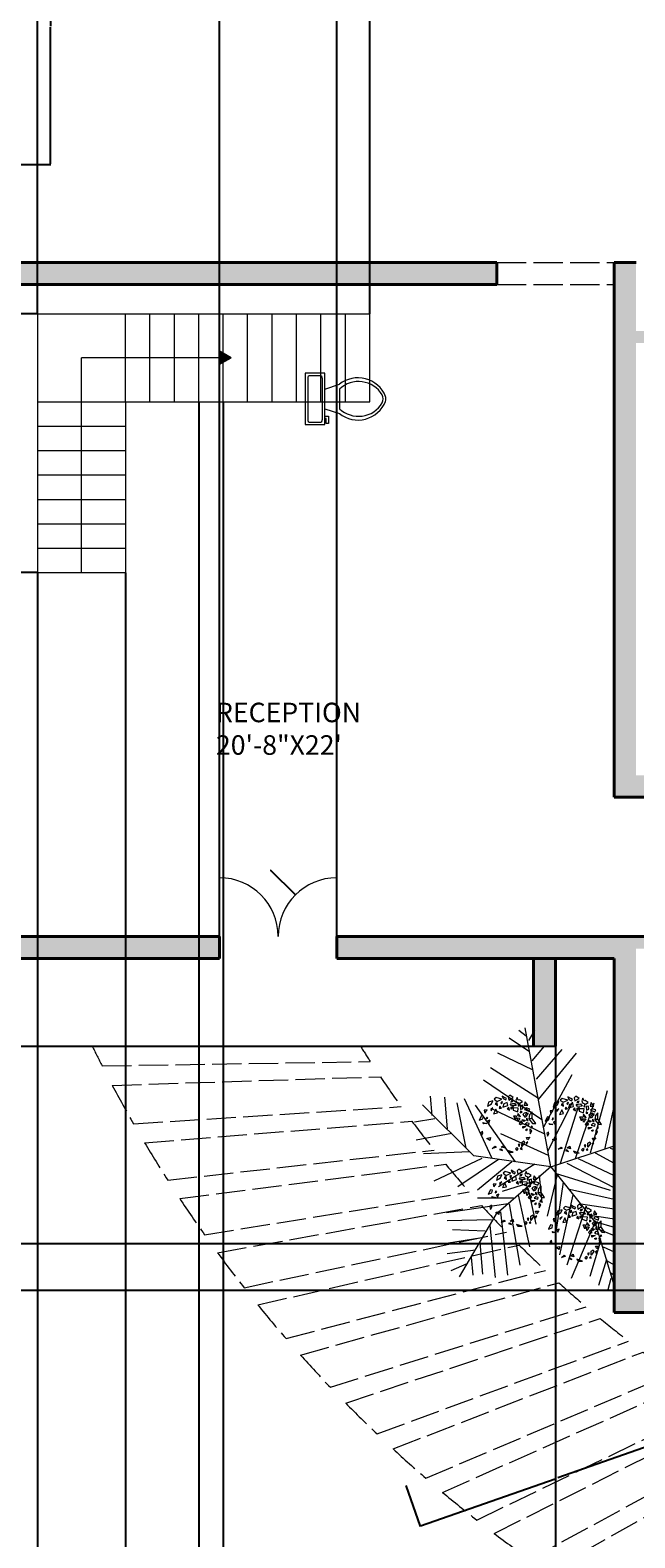
# Model space of a CAD drawing. Units: inches. Extents: x 2330 to 3943, y 1763 to 3461.
# Tile 11 of 40: x 2730 to 2977, y 2211 to 2829. Entities that reach past the tile are written whole.
import ezdxf

# ---------------------------------------------------------------- set-up
doc = ezdxf.new("R2010")
doc.units = ezdxf.units.IN
doc.linetypes.add('ACAD_ISO02W100', pattern=[15, 12, -3])
for name, color, linetype, lineweight in [('A-ANNO-DIMS', 2, 'Continuous', 18), ('A-AREA-IDEN', 7, 'Continuous', 18), ('A-DOOR', 4, 'Continuous', 18), ('A-FLOR', 7, 'Continuous', 25), ('A-FLOR-FIXT', 8, 'Continuous', 18), ('A-FLOR-STRS', 7, 'Continuous', 18), ('A-WALL', 7, 'Continuous', 40), ('A-WALL-OVHD', 7, 'ACAD_ISO02W100', 18), ('A-WALL-PATT', 252, 'Continuous', 13), ('L-PLNT', 94, 'Continuous', 13), ('L-PVMT-JOIN', 9, 'ACAD_ISO02W100', 13)]:
    doc.layers.add(name, color=color, linetype=linetype, lineweight=lineweight)
doc.styles.get("Standard").update_dxf_attribs({"font": 'arial.ttf'})
doc.dimstyles.get("Standard").update_dxf_attribs({"dimtxt": 0.18, "dimasz": 0.18, "dimexe": 0.18, "dimexo": 0.0625, "dimgap": 0.09, "dimtad": 0, "dimtih": 1, "dimtoh": 1, "dimdec": 4, "dimzin": 0, "dimdsep": 46, "dimtxsty": 'Standard', "dimcen": 0.09, "dimadec": 0, "dimazin": 0, "dimtfac": 1, "dimtdec": 4, "dimtofl": 0, "dimtmove": 0, "dimatfit": 3, "dimfxl": 1, "dimtolj": 1, "dimtzin": 0, "dimarcsym": 0})

# ---------------------------------------------------------------- blocks, each defined once
blk = doc.blocks.new('*U9')
for p, q in [((9.5, -6), (9.5, -2)), ((-10, -8.5), (-8, -8.5)), ((-10, -9.5), (-10, -8.5)), ((-7, -9.5), (-10, -9.5)), ((-8, -8.5), (-8, -8)), ((-7, -8), (-7, -9.5)), ((-4, -8), (-6, -14)), ((4, -8), (6, -14)), ((4, -14), (-4, -14))]:
    blk.add_line(p, q)
blk.add_lwpolyline([(10.5, -8), (10.5, 0), (-10.5, 0), (-10.5, -8)], close=True)
for points in [[(-9.5, -2), (-9.5, -6)], [(8.5, -1), (-8.5, -1)], [(-8.5, -7), (8.5, -7)]]:
    blk.add_lwpolyline(points)
for centre, radius, start, end in [((-8.62, -1.88), 0.884, 81.8699, 188.1301), ((-8.62, -6.12), 0.884, 171.8699, 278.1301), ((8.62, -1.88), 0.884, 351.8699, 98.1301), ((8.62, -6.12), 0.884, 261.8699, 8.1301), ((3.52, -21.58), 12.17, 141.46911, 247.97143), ((4.2, -21.82), 11.33, 136.36773, 238.94682), ((-3.52, -21.58), 12.17, 292.02843, 38.53071), ((-4.2, -21.82), 11.33, 301.05301, 43.63209), ((0, -27.88), 4, 245.73182, 294.26817), ((0, -29), 4, 254.86053, 285.13947)]:
    blk.add_arc(centre, radius, start, end)
blk = doc.blocks.new('*U13')
for points in [[(-5.78, 9.75), (-7.54, 9.23), (-8.01, 7.5), (-6.26, 8.45)], [(-5.78, 6.81), (-6.66, 6.21), (-6.52, 5.69)], [(-4.57, 6.38), (-5.45, 4.47), (-3.89, 4.82)], [(-4.43, 11.05), (-5.18, 10.36), (-3.96, 9.49), (-2.07, 10.36)], [(-4.84, 8.63), (-3.83, 7.85), (-4.03, 8.97)], [(-2.88, 7.5), (-3.15, 6.64), (-2.27, 6.72)], [(-1.94, 9.49), (-2.48, 8.97), (-2.27, 8.54), (-1.8, 9.06)], [(-2, 11.66), (-1.6, 10.62), (-0.52, 10.1), (-0.18, 10.62), (-0.79, 10.96)], [(0.02, 9.06), (-1.33, 8.54), (-1.73, 7.16), (0.29, 7.76)], [(0.76, 7.16), (0.09, 6.46), (1.1, 5.95)], [(1.24, 12), (0.56, 11.31), (0.76, 10.01), (2.52, 11.05)], [(1.37, 8.54), (3.13, 8.8), (3.8, 7.85), (1.91, 7.76)], [(2.59, 9.93), (1.84, 9.75), (1.64, 9.23), (2.32, 9.41)], [(1.71, 6.29), (1.71, 7.07), (2.65, 7.5), (2.11, 6.9)], [(2.52, 6.81), (2.52, 5.86), (4.41, 5.17), (4.61, 6.72)], [(4.14, 11.14), (3.6, 10.01), (4, 9.23), (5.22, 8.71), (6.3, 9.41), (5.08, 10.19), (4.61, 10.01)], [(4.61, 8.28), (4.54, 7.76), (4.95, 7.59), (4.95, 8.28)], [(6.43, 7.94), (5.49, 7.68), (5.56, 6.21), (6.5, 6.64)], [(7.45, 9.32), (7.11, 7.94), (8.52, 7.94)], [(7.85, 6.81), (7.18, 6.21), (9, 5.51), (9.33, 6.38)], [(-11.32, 1.79), (-9.83, 2.31), (-9.63, 3.44), (-10.44, 3.52)], [(-8.21, 0.41), (-9.43, 0.32), (-9.83, 0.84)], [(-8.14, 6.03), (-9.36, 5.95), (-9.02, 4.73)], [(-8.21, 3.09), (-8.48, 2.31), (-7.87, 2.57)], [(-7, 1.79), (-7.94, 1.53), (-7.47, 0.49)], [(3.53, 1.88), (2.86, 3.52), (3.8, 3.52)], [(4.41, 4.56), (4.27, 3.7), (5.49, 3.26)], [(4.27, 2.74), (5.29, 2.66), (4.41, 1.27)], [(5.83, 1.53), (5.02, 0.41), (5.49, -0.02), (6.5, 0.41)], [(5.49, 5.51), (5.42, 4.82), (6.16, 5.08)], [(7.51, 1.71), (6.91, 1.27), (6.23, 2.14)], [(8.12, 4.99), (7.11, 4.65), (6.5, 4.13), (7.38, 3.09), (8.12, 3.52), (7.65, 3.87)], [(8.12, 0.75), (7.51, 0.15), (8.93, -0.28), (9.13, 0.49)], [(8.19, 2.57), (7.92, 2.05), (8.66, 1.53)], [(8.73, 4.73), (8.19, 4.56), (8.39, 3.87), (8.59, 4.04)], [(10.28, 5.17), (9.2, 4.04), (9, 2.31), (10.48, 0.49), (11.76, 0.41), (10.35, 2.48), (9.33, 2.4), (10.28, 2.83)], [(-10.03, -2.71), (-10.64, -3.31), (-10.44, -4.44), (-9.9, -3.49)], [(-8.28, -5.73), (-6.79, -5.3), (-7, -6.51)], [(7.78, -0.8), (6.43, -1.5), (6.43, -0.72)], [(8.32, -1.75), (7.98, -2.53), (7.58, -2.1)], [(9.33, -5.13), (8.46, -6.25), (7.98, -5.22)], [(9.33, -1.75), (9.54, -3.74), (10.14, -2.53)], [(10.08, -0.63), (9.74, -1.32), (10.48, -0.89)], [(-4.84, -8.85), (-4.43, -9.45), (-5.99, -9.8)], [(-2.54, -10.06), (-3.02, -10.23), (-1.8, -10.67)], [(-2.34, -9.2), (-1.26, -8.5), (-0.99, -9.54)], [(0.22, -10.58), (0.83, -11.27), (2.59, -11.36)], [(4.07, -9.45), (3.53, -9.97), (4.07, -10.58), (4.61, -9.89)], [(5.29, -7.98), (4.61, -8.16), (5.02, -8.94)], [(6.03, -9.45), (5.42, -9.97), (6.16, -10.15)], [(6.1, -8.94), (6.16, -7.21), (6.91, -6.69), (7.24, -7.38)], [(8.05, -8.07), (8.59, -7.12), (7.92, -7.55)]]:
    blk.add_lwpolyline(points, close=True)
blk = doc.blocks.new('PAVER-RADIAL')
for p, q in [((0, 15.76), (109.7, 19.29)), ((8.7, 0), (118.23, 7.05))]:
    blk.add_line(p, q)
for radius, start, end in [(463.83, 213.96986, 215.81207), (559.83, 207.9852, 209.8274)]:
    blk.add_arc((494.37, 278.45), radius, start, end)
blk = doc.blocks.new('*D25')
at = {"layer": 'A-ANNO-DIMS', "color": 0, "lineweight": -2, "transparency": 16777216}
for p, q in [((2994.99, 2271.94), (3000.9, 2255.1)), ((3000.67, 2255.21), (2945.58, 2235.87)), ((2883.43, 2232.78), (2889.34, 2215.93)), ((2889.45, 2216.16), (2944.54, 2235.5))]:
    blk.add_line(p, q, dxfattribs=at)
at = {"layer": 'A-ANNO-DIMS', "color": 0, "transparency": 16777216}
for points in [[(3000.66, 2255.23), (3000.68, 2255.18), (3000.84, 2255.27)], [(2889.44, 2216.19), (2889.46, 2216.14), (2889.28, 2216.1)]]:
    blk.add_solid(points, dxfattribs=at)
at = {"layer": 'Defpoints', "color": 0, "transparency": 16777216}
for p in [(2994.96, 2272), (3000.84, 2255.27), (2883.41, 2232.84)]:
    blk.add_point(p, dxfattribs=at)
at = {"layer": 'A-ANNO-DIMS', "color": 0, "transparency": 16777216, "insert": (2945.06, 2235.69), "char_height": 0.18, "attachment_point": 5}
blk.add_mtext('\\A1;PAVER 118 TYP.', dxfattribs=at)
blk = doc.blocks.new('*D52')
at = {"layer": 'A-ANNO-DIMS', "color": 0, "lineweight": -2, "transparency": 16777216}
for p, q in [((2705.22, 2886.72), (2738.1, 2886.72)), ((2737.92, 2886.54), (2737.92, 2830.48)), ((2737.92, 2774.05), (2737.92, 2830.11)), ((2705.22, 2773.87), (2738.1, 2773.87))]:
    blk.add_line(p, q, dxfattribs=at)
at = {"layer": 'A-ANNO-DIMS', "color": 0, "transparency": 16777216}
for points in [[(2737.89, 2886.54), (2737.95, 2886.54), (2737.92, 2886.72)], [(2737.89, 2774.05), (2737.95, 2774.05), (2737.92, 2773.87)]]:
    blk.add_solid(points, dxfattribs=at)
at = {"layer": 'Defpoints', "color": 0, "transparency": 16777216}
for p in [(2705.15, 2886.72), (2737.92, 2886.72), (2705.15, 2773.87)]:
    blk.add_point(p, dxfattribs=at)
at = {"layer": 'A-ANNO-DIMS', "color": 0, "transparency": 16777216, "insert": (2737.92, 2830.3), "char_height": 0.18, "attachment_point": 5}
blk.add_mtext('\\A1;113', dxfattribs=at)
blk = doc.blocks.new('*D70')
at = {"layer": 'A-ANNO-DIMS', "color": 0, "lineweight": -2, "transparency": 16777216}
for p, q in [((2732.66, 2606.59), (2732.66, 1901.2)), ((2768.66, 2606.59), (2768.66, 1901.2)), ((2732.84, 1901.38), (2750.44, 1901.38)), ((2768.48, 1901.38), (2750.88, 1901.38))]:
    blk.add_line(p, q, dxfattribs=at)
at = {"layer": 'A-ANNO-DIMS', "color": 0, "transparency": 16777216}
for points in [[(2732.84, 1901.41), (2732.84, 1901.35), (2732.66, 1901.38)], [(2768.48, 1901.41), (2768.48, 1901.35), (2768.66, 1901.38)]]:
    blk.add_solid(points, dxfattribs=at)
at = {"layer": 'Defpoints', "color": 0, "transparency": 16777216}
for p in [(2732.66, 2606.65), (2768.66, 2606.65), (2768.66, 1901.38)]:
    blk.add_point(p, dxfattribs=at)
at = {"layer": 'A-ANNO-DIMS', "color": 0, "transparency": 16777216, "insert": (2750.66, 1901.38), "char_height": 0.18, "attachment_point": 5}
blk.add_mtext('\\A1;36', dxfattribs=at)
blk = doc.blocks.new('*D71')
at = {"layer": 'A-ANNO-DIMS', "color": 0, "lineweight": -2, "transparency": 16777216}
for p, q in [((2732.6, 2712.65), (2330.5, 2712.65)), ((2330.68, 2712.47), (2330.68, 2659.83)), ((2330.68, 2606.83), (2330.68, 2659.47)), ((2732.6, 2606.65), (2330.5, 2606.65))]:
    blk.add_line(p, q, dxfattribs=at)
at = {"layer": 'A-ANNO-DIMS', "color": 0, "transparency": 16777216}
for points in [[(2330.65, 2712.47), (2330.71, 2712.47), (2330.68, 2712.65)], [(2330.65, 2606.83), (2330.71, 2606.83), (2330.68, 2606.65)]]:
    blk.add_solid(points, dxfattribs=at)
at = {"layer": 'Defpoints', "color": 0, "transparency": 16777216}
for p in [(2330.68, 2712.65), (2732.66, 2712.65), (2732.66, 2606.65)]:
    blk.add_point(p, dxfattribs=at)
at = {"layer": 'A-ANNO-DIMS', "color": 0, "transparency": 16777216, "insert": (2330.68, 2659.65), "char_height": 0.18, "attachment_point": 5}
blk.add_mtext('\\A1;106', dxfattribs=at)
blk = doc.blocks.new('*D72')
at = {"layer": 'A-ANNO-DIMS', "color": 0, "lineweight": -2, "transparency": 16777216}
for p, q in [((2732.66, 2712.71), (2732.66, 3461.3)), ((2732.84, 3461.12), (2800.38, 3461.12)), ((2868.48, 3461.12), (2800.94, 3461.12)), ((2868.66, 2712.71), (2868.66, 3461.3))]:
    blk.add_line(p, q, dxfattribs=at)
at = {"layer": 'A-ANNO-DIMS', "color": 0, "transparency": 16777216}
for points in [[(2732.84, 3461.15), (2732.84, 3461.09), (2732.66, 3461.12)], [(2868.48, 3461.15), (2868.48, 3461.09), (2868.66, 3461.12)]]:
    blk.add_solid(points, dxfattribs=at)
at = {"layer": 'Defpoints', "color": 0, "transparency": 16777216}
for p in [(2868.66, 3461.12), (2732.66, 2712.65), (2868.66, 2712.65)]:
    blk.add_point(p, dxfattribs=at)
at = {"layer": 'A-ANNO-DIMS', "color": 0, "transparency": 16777216, "insert": (2800.66, 3461.12), "char_height": 0.18, "attachment_point": 5}
blk.add_mtext('\\A1;136', dxfattribs=at)
blk = doc.blocks.new('*D73')
at = {"layer": 'A-ANNO-DIMS', "color": 0, "lineweight": -2, "transparency": 16777216}
for p, q in [((2798.66, 2676.59), (2798.66, 1901.2)), ((2808.66, 2676.59), (2808.66, 1901.2)), ((2798.84, 1901.38), (2803.45, 1901.38)), ((2808.48, 1901.38), (2803.87, 1901.38))]:
    blk.add_line(p, q, dxfattribs=at)
at = {"layer": 'A-ANNO-DIMS', "color": 0, "transparency": 16777216}
for points in [[(2798.84, 1901.41), (2798.84, 1901.35), (2798.66, 1901.38)], [(2808.48, 1901.41), (2808.48, 1901.35), (2808.66, 1901.38)]]:
    blk.add_solid(points, dxfattribs=at)
at = {"layer": 'Defpoints', "color": 0, "transparency": 16777216}
for p in [(2798.66, 2676.65), (2808.66, 2676.65), (2808.66, 1901.38)]:
    blk.add_point(p, dxfattribs=at)
at = {"layer": 'A-ANNO-DIMS', "color": 0, "transparency": 16777216, "insert": (2803.66, 1901.38), "char_height": 0.18, "attachment_point": 5}
blk.add_mtext('\\A1;10', dxfattribs=at)
blk = doc.blocks.new('*D74')
at = {"layer": 'A-ANNO-DIMS', "color": 0, "lineweight": -2, "transparency": 16777216}
for p, q in [((2807.16, 2457.71), (2807.16, 3461.3)), ((2807.34, 3461.12), (2830.94, 3461.12)), ((2854.98, 3461.12), (2831.38, 3461.12)), ((2855.16, 2457.71), (2855.16, 3461.3))]:
    blk.add_line(p, q, dxfattribs=at)
at = {"layer": 'A-ANNO-DIMS', "color": 0, "transparency": 16777216}
for points in [[(2807.34, 3461.15), (2807.34, 3461.09), (2807.16, 3461.12)], [(2854.98, 3461.15), (2854.98, 3461.09), (2855.16, 3461.12)]]:
    blk.add_solid(points, dxfattribs=at)
at = {"layer": 'Defpoints', "color": 0, "transparency": 16777216}
for p in [(2855.16, 3461.12), (2807.16, 2457.65), (2855.16, 2457.65)]:
    blk.add_point(p, dxfattribs=at)
at = {"layer": 'A-ANNO-DIMS', "color": 0, "transparency": 16777216, "insert": (2831.16, 3461.12), "char_height": 0.18, "attachment_point": 5}
blk.add_mtext('\\A1;48', dxfattribs=at)
blk = doc.blocks.new('*D77')
at = {"layer": 'A-ANNO-DIMS', "color": 0, "lineweight": -2, "transparency": 16777216}
for p, q in [((2717.66, 2412.59), (2717.66, 1901.2)), ((2944.66, 2412.59), (2944.66, 1901.2)), ((2717.84, 1901.38), (2830.87, 1901.38)), ((2944.48, 1901.38), (2831.45, 1901.38))]:
    blk.add_line(p, q, dxfattribs=at)
at = {"layer": 'A-ANNO-DIMS', "color": 0, "transparency": 16777216}
for points in [[(2717.84, 1901.41), (2717.84, 1901.35), (2717.66, 1901.38)], [(2944.48, 1901.41), (2944.48, 1901.35), (2944.66, 1901.38)]]:
    blk.add_solid(points, dxfattribs=at)
at = {"layer": 'Defpoints', "color": 0, "transparency": 16777216}
for p in [(2717.66, 2412.65), (2944.66, 2412.65), (2944.66, 1901.38)]:
    blk.add_point(p, dxfattribs=at)
at = {"layer": 'A-ANNO-DIMS', "color": 0, "transparency": 16777216, "insert": (2831.16, 1901.38), "char_height": 0.18, "attachment_point": 5}
blk.add_mtext('\\A1;227', dxfattribs=at)
blk = doc.blocks.new('*D80')
at = {"layer": 'A-ANNO-DIMS', "color": 0, "lineweight": -2, "transparency": 16777216}
for p, q in [((3166.6, 2331.7), (2330.5, 2331.7)), ((2330.68, 2331.52), (2330.68, 2322.36)), ((2330.68, 2312.83), (2330.68, 2321.99)), ((3166.6, 2312.65), (2330.5, 2312.65))]:
    blk.add_line(p, q, dxfattribs=at)
at = {"layer": 'A-ANNO-DIMS', "color": 0, "transparency": 16777216}
for points in [[(2330.65, 2331.52), (2330.71, 2331.52), (2330.68, 2331.7)], [(2330.65, 2312.83), (2330.71, 2312.83), (2330.68, 2312.65)]]:
    blk.add_solid(points, dxfattribs=at)
at = {"layer": 'Defpoints', "color": 0, "transparency": 16777216}
for p in [(2330.68, 2331.7), (3166.66, 2331.7), (3166.66, 2312.65)]:
    blk.add_point(p, dxfattribs=at)
at = {"layer": 'A-ANNO-DIMS', "color": 0, "transparency": 16777216, "insert": (2330.68, 2322.18), "char_height": 0.18, "attachment_point": 5}
blk.add_mtext('\\A1;19.046', dxfattribs=at)
blk = doc.blocks.new('*D106')
at = {"layer": 'A-ANNO-DIMS', "color": 0, "lineweight": -2, "transparency": 16777216}
for p, q in [((2827.83, 2484.81), (2828.01, 2484.81)), ((2828.01, 2484.81), (2838.06, 2474.75)), ((2855.07, 2457.65), (2855.25, 2457.65)), ((2855.16, 2457.56), (2855.16, 2457.74))]:
    blk.add_line(p, q, dxfattribs=at)
at = {"layer": 'A-ANNO-DIMS', "color": 0, "transparency": 16777216}
blk.add_solid([(2838.08, 2474.77), (2838.04, 2474.73), (2838.19, 2474.62)], dxfattribs=at)
at = {"layer": 'Defpoints', "color": 0, "transparency": 16777216}
for p in [(2838.19, 2474.62), (2855.16, 2457.65)]:
    blk.add_point(p, dxfattribs=at)
at = {"layer": 'A-ANNO-DIMS', "color": 0, "transparency": 16777216, "insert": (2827.33, 2484.81), "char_height": 0.18, "attachment_point": 5}
blk.add_mtext('\\A1;2X R24', dxfattribs=at)

msp = doc.modelspace()

# ---------------------------------------------------------------- hatches: boundary and pattern name
at = {"layer": 'A-FLOR-STRS'}
h = msp.add_hatch(color=256, dxfattribs=at)
h.dxf.hatch_style = 1
h.paths.add_polyline_path([(2811.8629, 2694.6524), (2807.0594, 2697.4257), (2807.0594, 2691.8792)])
at = {"layer": 'A-WALL-PATT'}
h = msp.add_hatch(color=256, dxfattribs=at)
h.dxf.hatch_style = 1
h.paths.add_polyline_path([(2920.6605, 2733.6524), (2720.6605, 2733.6524), (2720.6605, 2775.6524), (2711.6605, 2775.6524), (2711.6605, 2733.6524), (2682.1605, 2733.6524), (2682.1605, 2728.6524), (2711.6605, 2728.6524), (2711.6605, 2596.1524), (2720.6605, 2596.1524), (2720.6605, 2724.6524), (2920.6605, 2724.6524)])
h = msp.add_hatch(color=256, dxfattribs=at)
h.dxf.hatch_style = 1
h.paths.add_polyline_path([(3203.7816, 2523.6524), (2977.6605, 2523.6524), (2977.6605, 2700.6524), (2981.6605, 2700.6524), (2981.6605, 2705.6524), (2977.6605, 2705.6524), (2977.6605, 2733.6524), (2968.6605, 2733.6524), (2968.6605, 2514.6524), (3023.6605, 2514.6524), (3023.6605, 2510.6524), (3028.6605, 2510.6524), (3028.6605, 2514.6524), (3203.7816, 2514.6524)])
h = msp.add_hatch(color=256, dxfattribs=at)
h.dxf.hatch_style = 1
h.paths.add_polyline_path([(2807.1605, 2457.6524), (2693.6605, 2457.6524), (2693.6605, 2448.6524), (2807.1605, 2448.6524)])
h = msp.add_hatch(color=256, dxfattribs=at)
h.dxf.hatch_style = 1
h.paths.add_polyline_path([(2977.6605, 2452.6524), (2981.6605, 2452.6524), (2981.6605, 2457.6524), (2968.6605, 2457.6524), (2855.1605, 2457.6524), (2855.1605, 2448.6524), (2968.6605, 2448.6524), (2968.6605, 2303.6524), (3175.6605, 2303.6524), (3175.6605, 2331.6982), (3166.6605, 2331.6982), (3166.6605, 2312.6524), (2977.6605, 2312.6524)])
h = msp.add_hatch(color=256, dxfattribs=at)
h.dxf.hatch_style = 1
h.paths.add_polyline_path([(2944.6605, 2448.6524), (2935.6605, 2448.6524), (2935.6605, 2412.6524), (2944.6605, 2412.6524)])

# ---------------------------------------------------------------- linework, layer by layer
at = {"layer": 'A-DOOR'}
for p, q in [((2807.1605, 2457.6524), (2807.1605, 2481.6524)), ((2855.1605, 2457.6524), (2855.1605, 2481.6524))]:
    msp.add_line(p, q, dxfattribs=at)
for centre, start, end in [((2807.1605, 2457.6524), 0, 90), ((2855.1605, 2457.6524), 90, 180)]:
    msp.add_arc(centre, 24, start, end, dxfattribs=at)
at = {"layer": 'A-FLOR'}
for p, q in [((2717.6605, 2412.6524), (2755.0816, 2412.6524)), ((2755.0816, 2412.6524), (2864.8379, 2412.6524)), ((2864.8379, 2412.6524), (2944.6605, 2412.6524))]:
    msp.add_line(p, q, dxfattribs=at)
at = {"layer": 'A-FLOR-STRS'}
for p, q in [((2732.6605, 2712.6524), (2732.6605, 2606.6524)), ((2732.6605, 2712.6524), (2868.6605, 2712.6524)), ((2768.6605, 2676.6524), (2768.6605, 2712.6524)), ((2778.6605, 2676.6524), (2778.6605, 2712.6524)), ((2788.6605, 2676.6524), (2788.6605, 2712.6524)), ((2798.6605, 2676.6524), (2798.6605, 2712.6524)), ((2808.6605, 2696.5013), (2808.6605, 2712.6524)), ((2818.6605, 2676.6524), (2818.6605, 2712.6524)), ((2828.6605, 2676.6524), (2828.6605, 2712.6524)), ((2838.6605, 2676.6524), (2838.6605, 2712.6524)), ((2848.6605, 2676.6524), (2848.6605, 2712.6524)), ((2858.6605, 2676.6524), (2858.6605, 2712.6524)), ((2868.6605, 2676.6524), (2868.6605, 2712.6524)), ((2750.6605, 2606.6524), (2750.6605, 2694.6524)), ((2807.0594, 2694.6524), (2750.6605, 2694.6524)), ((2808.6605, 2676.6524), (2808.6605, 2692.8036)), ((2732.6605, 2676.6524), (2768.6605, 2676.6524)), ((2768.6605, 2676.6524), (2768.6605, 2606.6524)), ((2768.6605, 2676.6524), (2868.6605, 2676.6524)), ((2732.6605, 2666.6524), (2768.6605, 2666.6524)), ((2732.6605, 2656.6524), (2768.6605, 2656.6524)), ((2732.6605, 2646.6524), (2768.6605, 2646.6524)), ((2732.6605, 2636.6524), (2768.6605, 2636.6524)), ((2732.6605, 2626.6524), (2768.6605, 2626.6524)), ((2732.6605, 2616.6524), (2768.6605, 2616.6524)), ((2732.6605, 2606.6524), (2768.6605, 2606.6524))]:
    msp.add_line(p, q, dxfattribs=at)
msp.add_lwpolyline([(2811.8629, 2694.6524), (2807.0594, 2697.4257), (2807.0594, 2691.8792)], close=True, dxfattribs=at)
at = {"layer": 'A-WALL'}
for p, q in [((2720.6605, 2733.6524), (2920.6605, 2733.6524)), ((2920.6605, 2733.6524), (2920.6605, 2724.6524)), ((2968.6605, 2733.6524), (2968.6605, 2514.6524)), ((2968.6605, 2733.6524), (2977.6605, 2733.6524)), ((2720.6605, 2724.6524), (2920.6605, 2724.6524)), ((2968.6605, 2514.6524), (3023.6605, 2514.6524)), ((2693.6605, 2457.6524), (2807.1605, 2457.6524)), ((2807.1605, 2448.6524), (2807.1605, 2457.6524)), ((2855.1605, 2448.6524), (2855.1605, 2457.6524)), ((2855.1605, 2457.6524), (2968.6605, 2457.6524)), ((2968.6605, 2457.6524), (2981.6605, 2457.6524)), ((2693.6605, 2448.6524), (2807.1605, 2448.6524)), ((2855.1605, 2448.6524), (2968.6605, 2448.6524)), ((2935.6605, 2448.6524), (2935.6605, 2412.6524)), ((2944.6605, 2448.6524), (2944.6605, 2412.6524)), ((2968.6605, 2448.6524), (2968.6605, 2303.6524)), ((2968.6605, 2303.6524), (3175.6605, 2303.6524))]:
    msp.add_line(p, q, dxfattribs=at)
at = {"layer": 'A-WALL-OVHD'}
for p, q in [((2920.6605, 2733.6524), (2968.6605, 2733.6524)), ((2920.6605, 2724.6524), (2968.6605, 2724.6524))]:
    msp.add_line(p, q, dxfattribs=at)
at = {"layer": 'L-PLNT'}
for p, q in [((2934.0488, 2410.3311), (2925.7168, 2415.9041)), ((2932.5998, 2416.8331), (2929.7018, 2419.1551)), ((2942.7858, 2363.1931), (2932.2858, 2420.1931)), ((2933.6868, 2414.9751), (2936.2228, 2419.1551)), ((2935.4978, 2402.9001), (2921.0078, 2409.8661)), ((2935.1358, 2406.6161), (2940.2078, 2412.6531)), ((2936.9468, 2399.1851), (2947.4528, 2411.2601)), ((2937.6718, 2390.8251), (2953.2488, 2409.8661)), ((2937.6718, 2391.2901), (2918.1098, 2403.8291)), ((2939.1208, 2382.4661), (2915.2118, 2398.7201)), ((2939.8448, 2379.6791), (2951.4378, 2401.0431)), ((2894.2008, 2384.3241), (2893.4768, 2392.2191)), ((2899.2728, 2391.7541), (2900.3588, 2378.7511)), ((2907.2418, 2391.2901), (2918.4718, 2367.1401)), ((2959.0448, 2368.9981), (2965.9278, 2394.5411)), ((2911.2858, 2367.6931), (2890.2858, 2388.6931)), ((2904.3438, 2389.4321), (2907.9668, 2370.8561)), ((2928.2528, 2365.2831), (2911.9518, 2388.5031)), ((2918.4718, 2387.1101), (2939.8448, 2376.8931)), ((2941.6568, 2369.9271), (2951.7998, 2389.8971)), ((2946.7278, 2364.8181), (2953.9728, 2387.5741)), ((2952.8868, 2366.6761), (2960.4938, 2389.4321)), ((2964.8408, 2370.3911), (2968.6605, 2388.02)), ((2895.2878, 2382.9301), (2886.9558, 2381.5371)), ((2902.1708, 2376.8931), (2887.6808, 2374.1061)), ((2922.0948, 2376.8931), (2941.6568, 2368.0691)), ((2942.7858, 2363.1931), (2968.6605, 2371.818)), ((2909.4158, 2369.4621), (2890.5788, 2368.5331)), ((2914.4868, 2366.6761), (2894.9258, 2357.3881)), ((2921.3698, 2366.2111), (2904.7068, 2355.0651)), ((2942.7858, 2363.1931), (2911.2858, 2367.6931)), ((2926.8038, 2365.2831), (2912.6758, 2353.6721)), ((2953.9728, 2366.6761), (2968.6605, 2359.7023)), ((2960.8558, 2368.9981), (2968.6605, 2364.7404)), ((2967.0148, 2370.8561), (2968.6605, 2370.4136)), ((2942.7858, 2363.1931), (2920.2858, 2343.6931)), ((2936.2228, 2364.3541), (2921.3698, 2355.0651)), ((2938.0338, 2359.7101), (2939.1208, 2348.5641)), ((2945.2788, 2360.1741), (2941.2948, 2342.9911)), ((2942.7858, 2363.1931), (2960.7858, 2340.6931)), ((2944.5548, 2360.6381), (2967.0148, 2353.6721)), ((2949.2638, 2364.8181), (2968.8258, 2354.6011)), ((2936.2228, 2357.3881), (2922.8188, 2353.2081)), ((2933.3248, 2354.6011), (2936.5848, 2339.7401)), ((2947.8148, 2356.9231), (2944.9168, 2337.4181)), ((2950.3508, 2354.1371), (2968.6605, 2349.9946)), ((2925.3548, 2348.0991), (2899.9968, 2344.3841)), ((2927.5288, 2350.4211), (2912.6758, 2350.4211)), ((2925.7168, 2348.0991), (2930.0648, 2323.0211)), ((2929.3398, 2351.8151), (2934.0488, 2330.4521)), ((2951.7998, 2351.8151), (2946.3658, 2327.2011)), ((2955.0598, 2348.0991), (2968.6605, 2346.0479)), ((2918.4718, 2341.5971), (2900.3588, 2341.1331)), ((2920.2858, 2343.6931), (2905.2858, 2318.1931)), ((2922.0948, 2344.8481), (2924.9928, 2318.8411)), ((2956.8708, 2346.2421), (2949.2638, 2323.0211)), ((2960.8558, 2340.6691), (2951.0748, 2317.4481)), ((2959.0448, 2343.4551), (2968.6605, 2341.8861)), ((2960.7858, 2340.6931), (2968.6605, 2314.4439)), ((2961.2188, 2340.6691), (2968.6605, 2338.4793)), ((2915.9368, 2336.9531), (2902.5328, 2337.4181)), ((2917.7478, 2339.2751), (2919.9208, 2317.9121)), ((2961.9428, 2337.8821), (2968.6605, 2335.1708)), ((2914.4868, 2334.1671), (2899.9968, 2331.8451)), ((2911.9518, 2329.0581), (2900.3588, 2327.6651)), ((2913.7628, 2332.3091), (2914.8498, 2319.3061)), ((2963.0298, 2332.7741), (2958.6828, 2318.3771)), ((2964.1168, 2330.4521), (2968.6605, 2328.431)), ((2908.3288, 2323.4851), (2901.8078, 2320.6991)), ((2910.1398, 2326.2721), (2910.8648, 2318.8411)), ((2965.5658, 2325.3431), (2962.3048, 2314.6611)), ((2965.5658, 2324.8791), (2968.6605, 2323.1432)), ((2967.3768, 2317.4481), (2965.9278, 2312.3391)), ((2967.3768, 2319.7701), (2968.6605, 2318.8986))]:
    msp.add_line(p, q, dxfattribs=at)
at = {"layer": 'L-PVMT-JOIN'}
msp.add_line((2759.1119, 2404.6054), (2868.8541, 2406.3698), dxfattribs=at)
for radius, start, end in [(559.831, 206.1429913, 207.0640944), (463.831, 212.1276532, 213.0487562)]:
    msp.add_arc((3257.6403, 2659.3212), radius, start, end, dxfattribs=at)

# ---------------------------------------------------------------- block references
at = {"layer": 'A-FLOR-FIXT', "rotation": 90}
msp.add_blockref('*U9', (2842.2365, 2677.7863), dxfattribs=at)
at = {"layer": 'L-PLNT'}
for p in [(2924.7971, 2380.5524), (2951.778, 2380.2195), (2928.4612, 2350.2622), (2953.1104, 2335.9492)]:
    msp.add_blockref('*U13', p, dxfattribs=at)
at = {"layer": 'L-PVMT-JOIN'}
msp.add_blockref('PAVER-RADIAL', (2763.271, 2380.867), dxfattribs=at)
for p, rotation in [((2777.2702, 2357.3572), 2.763309021725332), ((2792.3865, 2334.5496), 5.526618043451238), ((2808.5847, 2312.4972), 8.28992706517695), ((2825.8273, 2291.2515), 11.0532360870693), ((2844.0741, 2270.8617), 13.81654510862811), ((2863.2827, 2251.3753), 16.57985412887902), ((2883.4084, 2232.8376), 19.34316315207948), ((2904.4044, 2215.2918), 22.10647217380505), ((2926.2218, 2198.7785), 24.86978119553056), ((2948.81, 2183.3363), 27.63309021683611), ((2972.1164, 2169.001), 30.39639923898183)]:
    msp.add_blockref('PAVER-RADIAL', p, dxfattribs=dict(at, rotation=rotation))

# ---------------------------------------------------------------- texts
at = {"layer": 'A-AREA-IDEN', "insert": (2805.696, 2553.3663), "char_height": 8, "attachment_point": 1}
msp.add_mtext_dynamic_manual_height_columns('RECEPTION\\P20\'-8"X22\'', width=150.311776, gutter_width=12.5, heights=[0], dxfattribs=at)

# ---------------------------------------------------------------- dimensions: what is measured, and where the dimension line sits
at = {"layer": 'A-ANNO-DIMS'}
for base, p1, p2, picture, middle in [((2868.6605, 3461.1231), (2732.6605, 2712.6524), (2868.6605, 2712.6524), '*D72', (2800.6605, 3461.1231)), ((2855.1605, 3461.1231), (2807.1605, 2457.6524), (2855.1605, 2457.6524), '*D74', (2831.1605, 3461.1231)), ((2808.6605, 1901.3774), (2798.6605, 2676.6524), (2808.6605, 2676.6524), '*D73', (2803.6605, 1901.3774)), ((2768.6605, 1901.3774), (2732.6605, 2606.6524), (2768.6605, 2606.6524), '*D70', (2750.6605, 1901.3774)), ((2944.6605, 1901.3774), (2717.6605, 2412.6524), (2944.6605, 2412.6524), '*D77', (2831.1605, 1901.3774))]:
    dim = msp.add_linear_dim(base=base, p1=p1, p2=p2, dimstyle='Standard', override={"dimdec": 0, "dimlfac": 1, "dimrnd": 0, "dimzin": 0, "dimdsep": 46, "dimlunit": 2}, dxfattribs=at)
    dim.commit()
    dim.dimension.update_dxf_attribs({"geometry": picture, "text_midpoint": middle})
for base, p1, p2, override, picture, middle in [((2737.9166, 2886.7243), (2705.1545, 2773.8664), (2705.1545, 2886.7243), {"dimdec": 0, "dimlfac": 1, "dimrnd": 0, "dimzin": 0, "dimdsep": 46, "dimlunit": 2}, '*D52', (2737.9166, 2830.2954)), ((2330.6824, 2712.6524), (2732.6605, 2606.6524), (2732.6605, 2712.6524), {"dimdec": 0, "dimlfac": 1, "dimrnd": 0, "dimzin": 0, "dimdsep": 46, "dimlunit": 2}, '*D71', (2330.6824, 2659.6524)), ((2330.6824, 2331.6982), (3166.6605, 2312.6524), (3166.6605, 2331.6982), {"dimdec": 3, "dimlfac": 1, "dimrnd": 0, "dimzin": 0, "dimdsep": 46, "dimlunit": 2}, '*D80', (2330.6824, 2322.1753))]:
    dim = msp.add_linear_dim(base=base, p1=p1, p2=p2, angle=90, dimstyle='Standard', override=override, dxfattribs=at)
    dim.commit()
    dim.dimension.update_dxf_attribs({"geometry": picture, "text_midpoint": middle})
dim = msp.add_radius_dim(center=(2855.1605, 2457.6524), mpoint=(2838.19, 2474.623), text='2X <>', dimstyle='Standard', override={"dimdec": 0, "dimlfac": 1, "dimrnd": 0, "dimzin": 0, "dimdsep": 46, "dimlunit": 2}, dxfattribs=at)
dim.commit()
dim.dimension.update_dxf_attribs({"geometry": '*D106', "text_midpoint": (2827.328, 2484.8054), "dimtype": 164})
dim = msp.add_linear_dim(base=(3000.8384, 2255.2654), p1=(2883.4083, 2232.8381), p2=(2994.9643, 2271.9988), angle=19.3431632, text='PAVER <> TYP.', dimstyle='Standard', override={"dimdec": 0, "dimlfac": 1, "dimrnd": 0, "dimzin": 0, "dimdsep": 46, "dimlunit": 2}, dxfattribs=at)
dim.commit()
dim.dimension.update_dxf_attribs({"geometry": '*D25', "text_midpoint": (2945.0604, 2235.685)})

doc.saveas('drawing.dxf')
